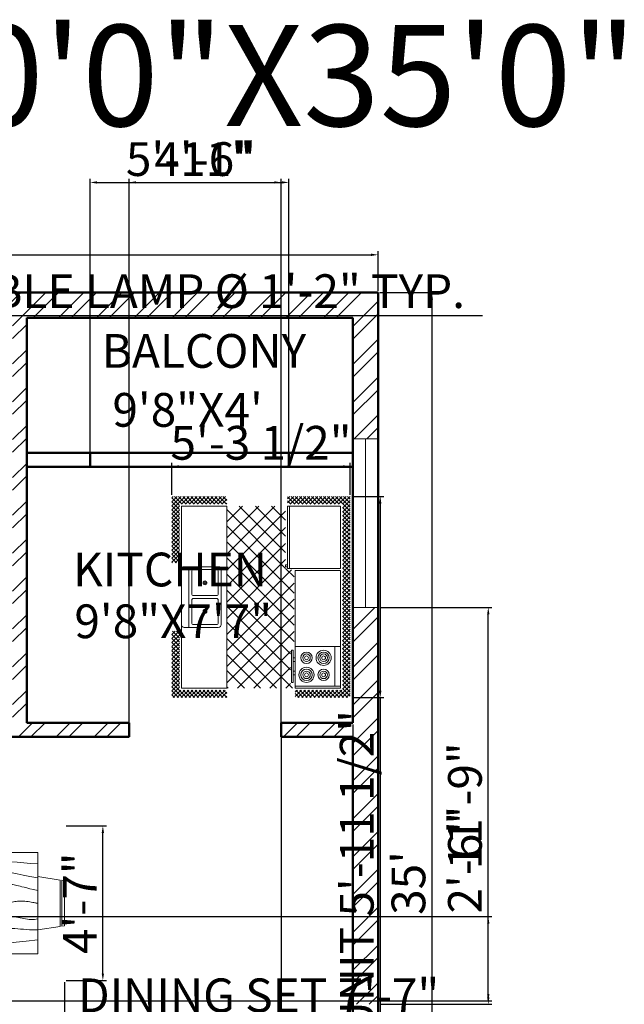
# Model space of a CAD drawing. Units: inches. Extents: x 1954 to 2815, y 1733 to 2371.
# Tile 4 of 4: x 2592 to 2807, y 2012 to 2362. Entities that reach past the tile are written whole.
import ezdxf

# ---------------------------------------------------------------- set-up
doc = ezdxf.new("R2010")
doc.units = ezdxf.units.IN
for name, color, linetype, lineweight in [('A-ANNO-DIMS', 2, 'Continuous', 18), ('A-ANNO-TEXT', 7, 'Continuous', 25), ('A-AREA-IDEN', 7, 'Continuous', 25), ('A-FLOR-FIXT', 9, 'Continuous', 20), ('A-FURN', 8, 'Continuous', 18), ('A-GLAZ', 4, 'Continuous', 18), ('A-WALL', 7, 'Continuous', 50), ('A-WALL-PATT', 252, 'Continuous', 13)]:
    doc.layers.add(name, color=color, linetype=linetype, lineweight=lineweight)
doc.styles.get("Standard").update_dxf_attribs({"font": 'arial.ttf'})
doc.dimstyles.new('ISO-25', dxfattribs={"dimtxt": 12, "dimasz": 2.5, "dimexe": 1.25, "dimexo": 0.625, "dimtad": 1, "dimdec": 1, "dimlunit": 4, "dimtxsty": 'Standard', "dimcen": 2.5, "dimadec": 0, "dimazin": 0, "dimtfac": 1, "dimtdec": 1, "dimtmove": 0, "dimatfit": 3, "dimfxl": 1, "dimarcsym": 0})

# ---------------------------------------------------------------- blocks, each defined once
blk = doc.blocks.new('Kitchen Layout - 7 x 8 ft')
for p, q in [((-5, 81.32), (2.68, 89)), ((-5, 83.44), (0.56, 89)), ((-5, 85.56), (-1.56, 89)), ((-5, 87.68), (-3.68, 89)), ((-1, 84.97), (-5, 88.97)), ((1.09, 85), (-2.91, 89)), ((3.21, 85), (-0.79, 89)), ((0.81, 85), (4.81, 89)), ((5.34, 85), (1.34, 89)), ((2.93, 85), (6.93, 89)), ((7.46, 85), (3.46, 89)), ((5.05, 85), (9.05, 89)), ((9.58, 85), (5.58, 89)), ((7.17, 85), (11.17, 89)), ((11.7, 85), (7.7, 89)), ((9.29, 85), (13.29, 89)), ((13.82, 85), (9.82, 89)), ((11.41, 85), (15.41, 89)), ((15.94, 85), (11.94, 89)), ((13.53, 85), (17.53, 89)), ((18.06, 85), (14.06, 89)), ((15.65, 85), (19.65, 89)), ((20.18, 85), (16.18, 89)), ((17.78, 85), (21.78, 89)), ((22.31, 85), (18.31, 89)), ((19.9, 85), (23.9, 89)), ((24.43, 85), (20.43, 89)), ((22.02, 85), (26.02, 89)), ((26.55, 85), (22.55, 89)), ((24.14, 85), (28.14, 89)), ((28.67, 85), (24.67, 89)), ((26.26, 85), (30.26, 89)), ((30.79, 85), (26.79, 89)), ((28.38, 85), (32.38, 89)), ((32.91, 85), (28.91, 89)), ((30.5, 85), (34.5, 89)), ((35.03, 85), (31.03, 89)), ((32.63, 85), (36.63, 89)), ((37.16, 85), (33.16, 89)), ((34.75, 85), (38.75, 89)), ((39.28, 85), (35.28, 89)), ((36.87, 85), (40.87, 89)), ((41.4, 85), (37.4, 89)), ((38.99, 85), (42.99, 89)), ((43.52, 85), (39.52, 89)), ((41.11, 85), (45.11, 89)), ((45.64, 85), (41.64, 89)), ((43.23, 85), (47.23, 89)), ((47.76, 85), (43.76, 89)), ((45.35, 85), (49.35, 89)), ((49.88, 85), (45.88, 89)), ((47.47, 85), (51.47, 89)), ((52, 85), (48, 89)), ((49.6, 85), (53.6, 89)), ((54.13, 85), (50.13, 89)), ((51.72, 85), (55.72, 89)), ((56.25, 85), (52.25, 89)), ((53.84, 85), (57.84, 89)), ((58.37, 85), (54.37, 89)), ((55.96, 85), (59.96, 89)), ((60.49, 85), (56.49, 89)), ((58.08, 85), (62.08, 89)), ((62.61, 85), (58.61, 89)), ((60.2, 85), (64.2, 89)), ((64.73, 85), (60.73, 89)), ((62.32, 85), (66.32, 89)), ((66.85, 85), (62.85, 89)), ((64.45, 85), (68.45, 89)), ((68.97, 85), (64.97, 89)), ((66.57, 85), (70.57, 89)), ((71.1, 85), (67.1, 89)), ((68.69, 85), (72.69, 89)), ((73.22, 85), (69.22, 89)), ((70.81, 85), (74.81, 89)), ((75.34, 85), (71.34, 89)), ((72.93, 85), (76.93, 89)), ((77.46, 85), (73.46, 89)), ((75.05, 85), (79.05, 89)), ((79.58, 85), (75.58, 89)), ((77.17, 85), (81.17, 89)), ((81.7, 85), (77.7, 89)), ((79.29, 85), (83.29, 89)), ((83.82, 85), (79.82, 89)), ((81.42, 85), (85.42, 89)), ((85.95, 85), (81.95, 89)), ((83.54, 85), (87.54, 89)), ((88.07, 85), (84.07, 89)), ((85.66, 85), (89.66, 89)), ((90.19, 85), (86.19, 89)), ((87.78, 85), (91.78, 89)), ((92.31, 85), (88.31, 89)), ((89.9, 85), (93.9, 89)), ((94.43, 85), (90.43, 89)), ((92.02, 85), (96.02, 89)), ((96.55, 85), (92.55, 89)), ((94.14, 85), (98.14, 89)), ((101, 82.67), (94.67, 89)), ((96.27, 85), (100.27, 89)), ((101, 84.79), (96.79, 89)), ((101, 86.92), (98.92, 89)), ((-1, 82.85), (-5, 86.85)), ((-1, 80.73), (-5, 84.73)), ((-5, 79.19), (-1, 83.19)), ((34, 84), (96, 84)), ((34, 60), (34, 84)), ((96, 84), (96, 60)), ((97, 83.61), (101, 87.61)), ((97, 81.49), (101, 85.49)), ((101, 80.55), (97, 84.55)), ((97, 79.37), (101, 83.37)), ((-1, 78.61), (-5, 82.61)), ((-5, 77.07), (-1, 81.07)), ((-1, 76.49), (-5, 80.49)), ((-5, 74.95), (-1, 78.95)), ((-1, 74.36), (-5, 78.36)), ((74, 81), (95, 81)), ((101, 78.43), (97, 82.43)), ((97, 77.25), (101, 81.25)), ((101, 76.31), (97, 80.31)), ((97, 75.13), (101, 79.13)), ((101, 74.19), (97, 78.19)), ((-5, 72.83), (-1, 76.83)), ((-1, 72.24), (-5, 76.24)), ((-5, 70.71), (-1, 74.71)), ((-1, 70.12), (-5, 74.12)), ((97, 73.01), (101, 77.01)), ((101, 72.07), (97, 76.07)), ((97, 70.89), (101, 74.89)), ((101, 69.95), (97, 73.95)), ((97, 68.76), (101, 72.76)), ((-5, 68.59), (-1, 72.59)), ((-1, 68), (-5, 72)), ((-5, 66.47), (-1, 70.47)), ((-1, 65.88), (-5, 69.88)), ((-5, 64.35), (-1, 68.35)), ((-1, 63.76), (-5, 67.76)), ((101, 67.82), (97, 71.82)), ((97, 66.64), (101, 70.64)), ((101, 65.7), (97, 69.7)), ((97, 64.52), (101, 68.52)), ((101, 63.58), (97, 67.58)), ((-5, 62.22), (-1, 66.22)), ((-1, 61.64), (-5, 65.64)), ((-5, 60.1), (-1, 64.1)), ((-1, 59.52), (-5, 63.52)), ((97, 62.4), (101, 66.4)), ((101, 61.46), (97, 65.46)), ((97, 60.28), (101, 64.28)), ((100.34, 60), (97, 63.34)), ((-5, 57.98), (-1, 61.98)), ((-1, 57.39), (-5, 61.39)), ((-1.73, 56), (-5, 59.27)), ((-3.85, 56), (-5, 57.15)), ((-4.86, 56), (-1, 59.86)), ((-2.74, 56), (-1, 57.74)), ((10.4, 24), (45.9, 59.5)), ((18.88, 24), (54.38, 59.5)), ((27.37, 24), (62.87, 59.5)), ((33.03, 55.11), (37.41, 59.5)), ((67.71, 24), (33.68, 58.04)), ((96, 60), (34, 60)), ((35.85, 24), (71.35, 59.5)), ((76.2, 24), (40.7, 59.5)), ((44.34, 24), (77.84, 57.5)), ((84.68, 24), (49.18, 59.5)), ((52.82, 24), (86.32, 57.5)), ((93.17, 24), (57.67, 59.5)), ((61.31, 24), (96, 58.69)), ((96, 29.65), (66.15, 59.5)), ((96, 38.14), (76.64, 57.5)), ((80, 60), (80, 59)), ((82, 59), (82, 60)), ((96, 46.63), (85.13, 57.5)), ((87, 59), (87, 60)), ((89, 60), (89, 59)), ((96, 55.11), (93.57, 57.54)), ((98.22, 60), (97, 61.22)), ((98.84, 60), (101, 62.16)), ((100.96, 60), (101, 60.04)), ((0, 57), (33, 57)), ((0, 30.57), (24.43, 55)), ((0, 39.06), (15.94, 55)), ((0, 47.54), (7.46, 55)), ((1.91, 24), (32.91, 55)), ((33.77, 24), (2.77, 55)), ((42.26, 24), (11.26, 55)), ((50.74, 24), (19.74, 55)), ((59.23, 24), (28.23, 55)), ((31, 55), (31, 56)), ((32, 55), (31, 55)), ((32, 56), (32, 55)), ((25.29, 24), (0, 49.29)), ((69.79, 24), (96, 50.21)), ((78.28, 24), (96, 41.72)), ((16.8, 24), (0, 40.8)), ((8.32, 24), (0, 32.32)), ((86.76, 24), (96, 33.24)), ((-5, 21.92), (-2.92, 24)), ((-5, 19.8), (-1, 23.8)), ((-1, 19.21), (-5, 23.21)), ((-5, 17.68), (-1, 21.68)), ((-1, 17.09), (-5, 21.09)), ((-1, 21.33), (-3.67, 24)), ((-1, 23.45), (-1.55, 24)), ((0, 24), (96, 24)), ((0, 0), (0, 24)), ((95.25, 24), (96, 24.75)), ((96, 24), (96, 0)), ((97, 22.1), (98.9, 24)), ((97, 19.97), (101, 23.97)), ((101, 19.03), (97, 23.03)), ((97, 17.85), (101, 21.85)), ((101, 16.91), (97, 20.91)), ((101, 21.16), (98.16, 24)), ((101, 23.28), (100.28, 24)), ((-5, 15.55), (-1, 19.55)), ((-1, 14.97), (-5, 18.97)), ((-5, 13.43), (-1, 17.43)), ((-1, 12.85), (-5, 16.85)), ((47.25, 6.5), (47.25, 18.5)), ((48.75, 18.5), (48.75, 6.5)), ((97, 15.73), (101, 19.73)), ((101, 14.79), (97, 18.79)), ((97, 13.61), (101, 17.61)), ((101, 12.67), (97, 16.67)), ((-5, 11.31), (-1, 15.31)), ((-1, 10.73), (-5, 14.73)), ((-5, 9.19), (-1, 13.19)), ((-1, 8.6), (-5, 12.6)), ((-5, 7.07), (-1, 11.07)), ((-1, 6.48), (-5, 10.48)), ((97, 11.49), (101, 15.49)), ((101, 10.55), (97, 14.55)), ((97, 9.37), (101, 13.37)), ((101, 8.43), (97, 12.43)), ((97, 7.25), (101, 11.25)), ((-5, 4.95), (-1, 8.95)), ((-1, 4.36), (-5, 8.36)), ((-5, 2.83), (-1, 6.83)), ((-1, 2.24), (-5, 6.24)), ((101, 6.31), (97, 10.31)), ((97, 5.12), (101, 9.12)), ((101, 4.18), (97, 8.18)), ((97, 3), (101, 7)), ((101, 2.06), (97, 6.06)), ((-5, 0.71), (-1, 4.71)), ((-1, 0.12), (-5, 4.12)), ((-5, -1.42), (-1, 2.58)), ((2, -5), (-5, 2)), ((-5, -3.54), (-1, 0.46)), ((96, 0), (0, 0)), ((64, 4), (32, 4)), ((93.24, -5), (101, 2.76)), ((95.36, -5), (101, 0.64)), ((97, 0.88), (101, 4.88)), ((101, -0.06), (97, 3.94)), ((101, -2.18), (97, 1.82)), ((-0.12, -5), (-5, -0.12)), ((-2.25, -5), (-5, -2.25)), ((-4.37, -5), (-5, -4.37)), ((-4.34, -5), (-0.34, -1)), ((-2.22, -5), (1.78, -1)), ((-0.1, -5), (3.9, -1)), ((4.12, -5), (0.12, -1)), ((2.02, -5), (6.02, -1)), ((6.24, -5), (2.24, -1)), ((4.14, -5), (8.14, -1)), ((8.36, -5), (4.36, -1)), ((6.27, -5), (10.27, -1)), ((10.48, -5), (6.48, -1)), ((8.39, -5), (12.39, -1)), ((12.6, -5), (8.6, -1)), ((10.51, -5), (14.51, -1)), ((14.73, -5), (10.73, -1)), ((12.63, -5), (16.63, -1)), ((16.85, -5), (12.85, -1)), ((14.75, -5), (18.75, -1)), ((18.97, -5), (14.97, -1)), ((16.87, -5), (20.87, -1)), ((21.09, -5), (17.09, -1)), ((18.99, -5), (22.99, -1)), ((23.21, -5), (19.21, -1)), ((21.11, -5), (25.11, -1)), ((25.33, -5), (21.33, -1)), ((23.24, -5), (27.24, -1)), ((27.45, -5), (23.45, -1)), ((25.36, -5), (29.36, -1)), ((29.57, -5), (25.57, -1)), ((27.48, -5), (30, -2.48)), ((30, -3.3), (27.7, -1)), ((29.6, -5), (30, -4.6)), ((30, -1.18), (29.82, -1)), ((66, -2.54), (67.54, -1)), ((66, -4.66), (69.66, -1)), ((69.88, -5), (66, -1.12)), ((67.76, -5), (66, -3.24)), ((67.78, -5), (71.78, -1)), ((72, -5), (68, -1)), ((69.9, -5), (73.9, -1)), ((74.12, -5), (70.12, -1)), ((72.03, -5), (76.03, -1)), ((76.24, -5), (72.24, -1)), ((74.15, -5), (78.15, -1)), ((78.36, -5), (74.36, -1)), ((76.27, -5), (80.27, -1)), ((80.49, -5), (76.49, -1)), ((78.39, -5), (82.39, -1)), ((82.61, -5), (78.61, -1)), ((80.51, -5), (84.51, -1)), ((84.73, -5), (80.73, -1)), ((82.63, -5), (86.63, -1)), ((86.85, -5), (82.85, -1)), ((84.75, -5), (88.75, -1)), ((88.97, -5), (84.97, -1)), ((86.88, -5), (90.88, -1)), ((91.09, -5), (87.09, -1)), ((89, -5), (93, -1)), ((93.21, -5), (89.21, -1)), ((91.12, -5), (95.12, -1)), ((95.34, -5), (91.34, -1)), ((97.46, -5), (93.46, -1)), ((99.58, -5), (95.58, -1)), ((101, -4.3), (97, -0.3)), ((97.48, -5), (101, -1.48)), ((99.6, -5), (101, -3.6))]:
    blk.add_line(p, q)
for points in [[(0, 56), (0, 84), (33, 84), (33, 56)], [(74, 60), (74, 84), (95, 84), (95, 60)], [(76, 58), (76, 59), (93, 59), (93, 58)]]:
    blk.add_lwpolyline(points, close=True)
for points in [[(33.5, 21), (62.5, 21)], [(32, 1.5), (32, 19.5)], [(33.5, 6.5), (33.5, 18.5)], [(34.5, 19.5), (46.25, 19.5)], [(49.75, 19.5), (61.5, 19.5)], [(62.5, 18.5), (62.5, 6.5)], [(64, 19.5), (64, 1.5)], [(46.25, 5.5), (34.5, 5.5)], [(61.5, 5.5), (49.75, 5.5)], [(62.5, 0), (33.5, 0)]]:
    blk.add_lwpolyline(points)
for centre, radius in [((80, 75), 4), ((80, 75), 3), ((89, 75), 3), ((80, 75), 2), ((80, 75), 1), ((89, 75), 2), ((89, 75), 1), ((80, 66), 3), ((80, 66), 2), ((89, 66), 4), ((89, 66), 3), ((89, 66), 2), ((80, 66), 1), ((89, 66), 1), ((40.5, 12.5), 1), ((40.5, 12.5), 0.5), ((55.5, 12.5), 1), ((55.5, 12.5), 0.5)]:
    blk.add_circle(centre, radius)
for centre, radius, start, end in [((33.5, 19.5), 1.5, 90, 180), ((62.5, 19.5), 1.5, 0, 90), ((34.5, 18.5), 1, 90, 180), ((46.25, 18.5), 1, 0, 90), ((49.75, 18.5), 1, 90, 180), ((61.5, 18.5), 1, 0, 90), ((34.5, 6.5), 1, 180, 270), ((46.25, 6.5), 1, 270, 0), ((49.75, 6.5), 1, 180, 270), ((61.5, 6.5), 1, 270, 0), ((33.5, 1.5), 1.5, 180, 270), ((62.5, 1.5), 1.5, 270, 0)]:
    blk.add_arc(centre, radius, start, end)
blk = doc.blocks.new('Dining Set - 36 x 72 in.')
for p, q in [((-22.2343, 26.00059), (-23.4847, 17.99762)), ((-22.2304, 26), (-5.7608, 26)), ((-22, 27.5), (-22.1562, 26.50042)), ((-5.8416, 26.5), (-22.1534, 26.5)), ((-22, 27.5), (-6, 27.5)), ((-5.8437, 26.49966), (-6, 27.5)), ((-4.5152, 17.99762), (-5.7655, 25.99926)), ((5.7657, 26.00059), (4.5153, 17.99762)), ((5.7696, 26), (22.2392, 26)), ((6, 27.5), (5.8438, 26.50042)), ((22.1584, 26.5), (5.8466, 26.5)), ((6, 27.5), (22, 27.5)), ((22.1563, 26.49966), (22, 27.5)), ((23.4848, 17.99762), (22.2345, 25.99926)), ((36, 18), (-36, 18)), ((-36, 18), (-36, -18)), ((36, -18), (36, 18)), ((-45.5, 8), (-44.5004, 8.15617)), ((-45.5, 8), (-45.5, -8)), ((-44.5, -8.15843), (-44.5, 8.15338)), ((-44.0006, 8.23428), (-35.9976, 9.48474)), ((-44, 8.23041), (-44, -8.23915)), ((44.0006, 8.23428), (35.9976, 9.48474)), ((44, 8.23041), (44, -8.23915)), ((44.5, -8.15843), (44.5, 8.15338)), ((45.5, 8), (44.5005, 8.15617)), ((45.5, 8), (45.5, -8)), ((-44.4997, -8.15631), (-45.5, -8)), ((-35.9976, -9.48476), (-43.9993, -8.2345)), ((35.9976, -9.48476), (43.9993, -8.2345)), ((44.4997, -8.15631), (45.5, -8)), ((-36, -18), (36, -18)), ((-22.2343, -26.0006), (-23.4847, -17.99762)), ((-4.5152, -17.99762), (-5.7655, -25.99928)), ((5.7657, -26.0006), (4.5153, -17.99762)), ((23.4848, -17.99762), (22.2345, -25.99928)), ((-22.2304, -26), (-5.7608, -26)), ((-22, -27.5), (-22.1562, -26.50044)), ((-5.8416, -26.5), (-22.1534, -26.5)), ((-22, -27.5), (-6, -27.5)), ((-5.8437, -26.49967), (-6, -27.5)), ((5.7696, -26), (22.2392, -26)), ((6, -27.5), (5.8438, -26.50044)), ((22.1584, -26.5), (5.8466, -26.5)), ((6, -27.5), (22, -27.5)), ((22.1563, -26.49967), (22, -27.5))]:
    blk.add_line(p, q)
for points in [[(-36, 15), (-31.1772, 14.97754), (-26.8079, 14.91406), (-22.8538, 14.81543), (-19.276, 14.6875), (-16.0362, 14.53613), (-13.0957, 14.36718), (-10.4159, 14.18652), (-7.9583, 14), (-5.6904, 13.81315), (-3.6035, 13.63021), (-1.6954, 13.45508), (0.0365, 13.29166), (1.5945, 13.14388), (2.9811, 13.01562), (4.1988, 12.9108), (5.25, 12.83333), (6.1393, 12.78613), (6.8802, 12.76823), (7.4883, 12.77767), (7.9792, 12.8125), (8.3685, 12.87077), (8.6719, 12.95052), (8.9049, 13.0498), (9.0833, 13.16666), (9.2205, 13.29899), (9.3216, 13.44401), (9.3895, 13.59879), (9.4271, 13.76041), (9.4373, 13.92594), (9.4232, 14.09245), (9.3875, 14.257), (9.3333, 14.41666), (9.2638, 14.56917), (9.1836, 14.71484), (9.0975, 14.85465), (9.0104, 14.98958), (8.9272, 15.1206), (8.8529, 15.2487), (8.7922, 15.37483), (8.75, 15.5), (8.7305, 15.62467), (8.7344, 15.74739), (8.7617, 15.86621), (8.8125, 15.97916), (8.8867, 16.08431), (8.9844, 16.17968), (9.1055, 16.26334), (9.25, 16.33333), (9.4189, 16.38802), (9.6172, 16.42708), (9.8506, 16.45052), (10.125, 16.45833), (10.4463, 16.45052), (10.8203, 16.42708), (11.2529, 16.38802), (11.75, 16.33333), (12.3184, 16.26318), (12.9694, 16.17838), (13.7151, 16.07991), (14.5677, 15.96875), (15.5395, 15.84586), (16.6426, 15.71224), (17.8893, 15.56884), (19.2917, 15.41666), (20.859, 15.25667), (22.5879, 15.08984), (24.4721, 14.91715), (26.5052, 14.73958), (28.6809, 14.5581), (30.9929, 14.3737), (33.4347, 14.18733), (36, 14)], [(-36, 10), (-28.9766, 10.14274), (-23.1725, 10.20442), (-18.4241, 10.19775), (-14.5677, 10.13541), (-11.4399, 10.03011), (-8.877, 9.89453), (-6.7154, 9.74137), (-4.7917, 9.58333), (-2.9698, 9.43082), (-1.2246, 9.28515), (0.4415, 9.14534), (2.026, 9.01041), (3.5266, 8.87939), (4.9408, 8.7513), (6.266, 8.62516), (7.5, 8.5), (8.6411, 8.37549), (9.6914, 8.2539), (10.6538, 8.13818), (11.5312, 8.03125), (12.3267, 7.93603), (13.043, 7.85547), (13.6831, 7.79248), (14.25, 7.75), (14.7471, 7.7303), (15.1797, 7.73307), (15.5537, 7.75732), (15.875, 7.80208), (16.1494, 7.86637), (16.3828, 7.94922), (16.5811, 8.04964), (16.75, 8.16666), (16.8944, 8.29915), (17.0143, 8.44531), (17.1089, 8.60319), (17.1771, 8.77083), (17.218, 8.94629), (17.2305, 9.1276), (17.2137, 9.31282), (17.1667, 9.5), (17.0895, 9.6875), (16.987, 9.875), (16.8649, 10.0625), (16.7292, 10.25), (16.5856, 10.4375), (16.4401, 10.625), (16.2985, 10.8125), (16.1667, 11), (16.05, 11.18733), (15.9518, 11.3737), (15.8752, 11.5581), (15.8229, 11.73958), (15.798, 11.91715), (15.8034, 12.08984), (15.842, 12.25667), (15.9167, 12.41666), (16.0295, 12.56836), (16.1784, 12.70833), (16.3605, 12.83268), (16.5729, 12.9375), (16.8127, 13.01888), (17.0768, 13.07291), (17.3625, 13.0957), (17.6667, 13.08333), (17.9894, 13.03312), (18.3418, 12.94726), (18.7382, 12.82918), (19.1927, 12.68229), (19.7195, 12.51001), (20.3327, 12.31575), (21.0465, 12.10294), (21.875, 11.875), (22.8357, 11.63354), (23.959, 11.37304), (25.2786, 11.08618), (26.8282, 10.76562), (28.6414, 10.40405), (30.752, 9.99414), (33.1936, 9.52856), (36, 9)], [(-36, 5.5), (-30.7157, 5.3348), (-26.069, 5.20963), (-21.9946, 5.11767), (-18.4271, 5.05208), (-15.3009, 5.00602), (-12.5508, 4.97265), (-10.1112, 4.94515), (-7.9167, 4.91666), (-5.909, 4.88167), (-4.0586, 4.83984), (-2.3429, 4.79215), (-0.7396, 4.73958), (0.7739, 4.6831), (2.22, 4.6237), (3.6213, 4.56233), (5, 4.5), (6.373, 4.43782), (7.7344, 4.3776), (9.0723, 4.32129), (10.375, 4.27083), (11.6309, 4.22819), (12.8281, 4.19531), (13.9551, 4.17415), (15, 4.16666), (15.954, 4.17448), (16.819, 4.19791), (17.6001, 4.23698), (18.3021, 4.29166), (18.9299, 4.36198), (19.4883, 4.44791), (19.9823, 4.54948), (20.4167, 4.66666), (20.7969, 4.79899), (21.1302, 4.94401), (21.4245, 5.09879), (21.6875, 5.26041), (21.9271, 5.42594), (22.1511, 5.59245), (22.3672, 5.757), (22.5834, 5.91666), (22.8065, 6.06868), (23.0404, 6.21093), (23.2879, 6.34147), (23.5521, 6.45833), (23.8358, 6.55957), (24.142, 6.64323), (24.4735, 6.70735), (24.8334, 6.75), (25.2235, 6.76969), (25.642, 6.76692), (26.0858, 6.74267), (26.5521, 6.69791), (27.0379, 6.63362), (27.5404, 6.55078), (28.0565, 6.45036), (28.5834, 6.33333), (29.1242, 6.19987), (29.7071, 6.04687), (30.3661, 5.87044), (31.1354, 5.66666), (32.0493, 5.43164), (33.142, 5.16146), (34.4475, 4.85221), (36, 4.5)], [(-36, -1), (-30.7915, -0.6591), (-26.0195, -0.38216), (-21.6519, -0.16284), (-17.6563, 0.00521), (-14.0005, 0.12833), (-10.6523, 0.21289), (-7.5796, 0.26522), (-4.75, 0.29166), (-2.134, 0.29793), (0.2878, 0.28711), (2.5317, 0.26163), (4.6146, 0.22396), (6.5529, 0.17651), (8.3633, 0.12174), (10.0623, 0.06209), (11.6667, 0), (13.1899, -0.06201), (14.6341, -0.1211), (15.9982, -0.17432), (17.2813, -0.21875), (18.4823, -0.25147), (19.6003, -0.26953), (20.6343, -0.27002), (21.5834, -0.25), (22.4481, -0.20768), (23.2357, -0.14584), (23.9549, -0.06836), (24.6146, 0.02083), (25.2235, 0.11784), (25.7904, 0.21875), (26.3241, 0.31966), (26.8334, 0.41666), (27.3265, 0.50618), (27.8099, 0.58593), (28.2894, 0.65397), (28.7709, 0.70833), (29.2601, 0.74707), (29.763, 0.76823), (30.2855, 0.76985), (30.8334, 0.75), (31.4088, 0.70784), (31.9994, 0.64713), (32.589, 0.57275), (33.1615, 0.48958), (33.7008, 0.4025), (34.1908, 0.3164), (34.6153, 0.23616), (34.9584, 0.16666), (35.2099, 0.11165), (35.3848, 0.07031), (35.504, 0.04069), (35.5886, 0.02083), (35.6594, 0.00879), (35.7377, 0.0026), (35.8442, 0.00032), (36, 0)], [(-36, -6.5), (-27.1843, -6.31267), (-20.084, -6.1263), (-14.469, -5.9419), (-10.1094, -5.76042), (-6.7752, -5.58285), (-4.2363, -5.41016), (-2.2629, -5.24333), (-0.625, -5.08334), (0.8708, -4.93099), (2.2715, -4.78646), (3.5872, -4.64974), (4.8281, -4.52084), (6.0046, -4.39974), (7.127, -4.28646), (8.2053, -4.18099), (9.25, -4.08334), (10.2705, -3.99382), (11.2734, -3.91407), (12.2647, -3.84603), (13.25, -3.79167), (14.2354, -3.75293), (15.2266, -3.73177), (16.2295, -3.73015), (17.25, -3.75), (18.2912, -3.79248), (19.3451, -3.85547), (20.4009, -3.93604), (21.4479, -4.03125), (22.4754, -4.13819), (23.4727, -4.25391), (24.4289, -4.37549), (25.3334, -4.5), (26.1785, -4.62492), (26.9694, -4.74935), (27.7145, -4.87281), (28.4219, -4.99479), (29.1, -5.11483), (29.7572, -5.23242), (30.4016, -5.34709), (31.0417, -5.45834), (31.6837, -5.56437), (32.3262, -5.65821), (32.9658, -5.73153), (33.599, -5.77604), (34.2224, -5.78345), (34.8327, -5.74545), (35.4264, -5.65373), (36, -5.5)], [(-36, -10), (-26.4022, -9.81299), (-18.4675, -9.62891), (-11.9839, -9.45069), (-6.7396, -9.28125), (-2.5226, -9.12354), (0.8789, -8.98047), (3.6769, -8.85498), (6.0833, -8.75), (8.2767, -8.66765), (10.3021, -8.60677), (12.1712, -8.56543), (13.8958, -8.54167), (15.4876, -8.53353), (16.9583, -8.53907), (18.3197, -8.55632), (19.5834, -8.58334), (20.7616, -8.61841), (21.8685, -8.66081), (22.9188, -8.71004), (23.9271, -8.76563), (24.9081, -8.82707), (25.8763, -8.89388), (26.8465, -8.96558), (27.8334, -9.04167), (28.8474, -9.12118), (29.8828, -9.20117), (30.93, -9.27824), (31.9792, -9.34896), (33.0205, -9.40991), (34.0443, -9.45768), (35.0407, -9.48885), (36, -9.5)], [(-36, -14.5), (-30.0881, -14.33513), (-25.0332, -14.21224), (-20.7312, -14.12647), (-17.0781, -14.07292), (-13.97, -14.04671), (-11.3027, -14.04297), (-8.9724, -14.05681), (-6.875, -14.08334), (-4.9224, -14.11833), (-3.0905, -14.16016), (-1.3709, -14.20785), (0.2448, -14.26042), (1.7647, -14.3169), (3.1973, -14.3763), (4.5507, -14.43767), (5.8333, -14.5), (7.0554, -14.5621), (8.235, -14.62175), (9.3922, -14.67652), (10.5469, -14.72396), (11.7192, -14.76164), (12.929, -14.78711), (14.1965, -14.79794), (15.5417, -14.79167), (16.9933, -14.76424), (18.6152, -14.70508), (20.4804, -14.60197), (22.6615, -14.44271), (25.2312, -14.21509), (28.2624, -13.9069), (31.8277, -13.50594), (36, -13)]]:
    blk.add_lwpolyline(points)
blk = doc.blocks.new('*D10')
at = {"layer": 'A-ANNO-DIMS', "color": 0, "lineweight": -2, "transparency": 16777216}
for p, q in [((2239.88, 2265.61), (2239.88, 2279.68)), ((2242.38, 2278.43), (2717.38, 2278.43)), ((2719.88, 2265.61), (2719.88, 2279.68))]:
    blk.add_line(p, q, dxfattribs=at)
at = {"layer": 'A-ANNO-DIMS', "color": 0, "transparency": 16777216}
for points in [[(2242.38, 2278.85), (2242.38, 2278.01), (2239.88, 2278.43)], [(2717.38, 2278.85), (2717.38, 2278.01), (2719.88, 2278.43)]]:
    blk.add_solid(points, dxfattribs=at)
at = {"layer": 'Defpoints', "color": 0, "transparency": 16777216}
for p in [(2719.88, 2278.43), (2239.88, 2264.98), (2719.88, 2264.98)]:
    blk.add_point(p, dxfattribs=at)
at = {"layer": 'A-ANNO-DIMS', "color": 0, "transparency": 16777216, "insert": (2479.88, 2285.18), "char_height": 12, "attachment_point": 5}
blk.add_mtext("40'", dxfattribs=at)
blk = doc.blocks.new('*D11')
at = {"layer": 'A-ANNO-DIMS', "color": 0, "lineweight": -2, "transparency": 16777216}
for p, q in [((2720.51, 2264.98), (2740.24, 2264.98)), ((2738.99, 2262.48), (2738.99, 1847.48)), ((2720.51, 1844.98), (2740.24, 1844.98))]:
    blk.add_line(p, q, dxfattribs=at)
at = {"layer": 'A-ANNO-DIMS', "color": 0, "transparency": 16777216}
for points in [[(2738.57, 2262.48), (2739.41, 2262.48), (2738.99, 2264.98)], [(2738.57, 1847.48), (2739.41, 1847.48), (2738.99, 1844.98)]]:
    blk.add_solid(points, dxfattribs=at)
at = {"layer": 'Defpoints', "color": 0, "transparency": 16777216}
for p in [(2719.88, 2264.98), (2719.88, 1844.98), (2738.99, 1844.98)]:
    blk.add_point(p, dxfattribs=at)
at = {"layer": 'A-ANNO-DIMS', "color": 0, "transparency": 16777216, "insert": (2732.23, 2054.98), "char_height": 12, "attachment_point": 5, "rotation": 90}
blk.add_mtext("35'", dxfattribs=at)
blk = doc.blocks.new('WIN-60IN')
blk.add_line((4.5, 60), (4.5, 0))
blk.add_lwpolyline([(9, 60), (9, 0), (0, 0), (0, 60)], close=True)
blk = doc.blocks.new('*D16')
at = {"layer": 'A-ANNO-DIMS', "color": 0, "lineweight": -2, "transparency": 16777216}
for p, q in [((2540.09, 2255.38), (2540.09, 2258.1)), ((2542.59, 2256.85), (2551.59, 2256.85)), ((2554.09, 2255.38), (2554.09, 2258.1)), ((2554.09, 2256.85), (2757.06, 2256.85))]:
    blk.add_line(p, q, dxfattribs=at)
at = {"layer": 'A-ANNO-DIMS', "color": 0, "transparency": 16777216}
for points in [[(2542.59, 2257.27), (2542.59, 2256.44), (2540.09, 2256.85)], [(2551.59, 2257.27), (2551.59, 2256.44), (2554.09, 2256.85)]]:
    blk.add_solid(points, dxfattribs=at)
at = {"layer": 'Defpoints', "color": 0, "transparency": 16777216}
for p in [(2554.09, 2256.85), (2540.09, 2254.75), (2554.09, 2254.75)]:
    blk.add_point(p, dxfattribs=at)
at = {"layer": 'A-ANNO-DIMS', "color": 0, "transparency": 16777216, "insert": (2656.83, 2263.94), "char_height": 12, "attachment_point": 5}
blk.add_mtext('TABLE LAMP Ø 1\'-2" TYP.', dxfattribs=at)
blk = doc.blocks.new('*D22')
at = {"layer": 'A-ANNO-DIMS', "color": 0, "lineweight": -2, "transparency": 16777216}
for p, q in [((2710.56, 2192.43), (2721.92, 2192.43)), ((2720.67, 2189.93), (2720.67, 2123.41)), ((2710.56, 2120.91), (2721.92, 2120.91)), ((2720.67, 2120.91), (2720.67, 1926.5))]:
    blk.add_line(p, q, dxfattribs=at)
at = {"layer": 'A-ANNO-DIMS', "color": 0, "transparency": 16777216}
for points in [[(2720.25, 2189.93), (2721.08, 2189.93), (2720.67, 2192.43)], [(2720.25, 2123.41), (2721.08, 2123.41), (2720.67, 2120.91)]]:
    blk.add_solid(points, dxfattribs=at)
at = {"layer": 'Defpoints', "color": 0, "transparency": 16777216}
for p in [(2709.94, 2192.43), (2709.94, 2120.91), (2720.67, 2120.91)]:
    blk.add_point(p, dxfattribs=at)
at = {"layer": 'A-ANNO-DIMS', "color": 0, "transparency": 16777216, "insert": (2713.84, 2022.46), "char_height": 12, "attachment_point": 5, "rotation": 90}
blk.add_mtext('KITCHEN UNIT 5\'-11 1/2"', dxfattribs=at)
blk = doc.blocks.new('*D23')
at = {"layer": 'A-ANNO-DIMS', "color": 0, "lineweight": -2, "transparency": 16777216}
for p, q in [((2646.51, 2193.06), (2646.51, 2204.41)), ((2709.94, 2193.06), (2709.94, 2204.41)), ((2649.01, 2203.16), (2707.44, 2203.16))]:
    blk.add_line(p, q, dxfattribs=at)
at = {"layer": 'A-ANNO-DIMS', "color": 0, "transparency": 16777216}
for points in [[(2649.01, 2203.58), (2649.01, 2202.75), (2646.51, 2203.16)], [(2707.44, 2203.58), (2707.44, 2202.75), (2709.94, 2203.16)]]:
    blk.add_solid(points, dxfattribs=at)
at = {"layer": 'Defpoints', "color": 0, "transparency": 16777216}
for p in [(2709.94, 2203.16), (2646.51, 2192.43), (2709.94, 2192.43)]:
    blk.add_point(p, dxfattribs=at)
at = {"layer": 'A-ANNO-DIMS', "color": 0, "transparency": 16777216, "insert": (2678.23, 2210), "char_height": 12, "attachment_point": 5}
blk.add_mtext('5\'-3 1/2"', dxfattribs=at)
blk = doc.blocks.new('*D24')
at = {"layer": 'A-ANNO-DIMS', "color": 0, "lineweight": -2, "transparency": 16777216}
for p, q in [((2517.32, 2019.64), (2517.32, 2005.36)), ((2608.32, 2019.64), (2608.32, 2005.36)), ((2519.82, 2006.61), (2605.82, 2006.61)), ((2608.32, 2006.61), (2743.97, 2006.61))]:
    blk.add_line(p, q, dxfattribs=at)
at = {"layer": 'A-ANNO-DIMS', "color": 0, "transparency": 16777216}
for points in [[(2519.82, 2007.03), (2519.82, 2006.2), (2517.32, 2006.61)], [(2605.82, 2007.03), (2605.82, 2006.2), (2608.32, 2006.61)]]:
    blk.add_solid(points, dxfattribs=at)
at = {"layer": 'Defpoints', "color": 0, "transparency": 16777216}
for p in [(2517.32, 2020.26), (2608.32, 2020.26), (2608.32, 2006.61)]:
    blk.add_point(p, dxfattribs=at)
at = {"layer": 'A-ANNO-DIMS', "color": 0, "transparency": 16777216, "insert": (2677.39, 2013.44), "char_height": 12, "attachment_point": 5}
blk.add_mtext('DINING SET 7\'-7"', dxfattribs=at)
blk = doc.blocks.new('*D25')
at = {"layer": 'A-ANNO-DIMS', "color": 0, "lineweight": -2, "transparency": 16777216}
for p, q in [((2608.95, 2075.26), (2623.22, 2075.26)), ((2621.97, 2022.76), (2621.97, 2072.76)), ((2608.95, 2020.26), (2623.22, 2020.26))]:
    blk.add_line(p, q, dxfattribs=at)
at = {"layer": 'A-ANNO-DIMS', "color": 0, "transparency": 16777216}
for points in [[(2621.56, 2072.76), (2622.39, 2072.76), (2621.97, 2075.26)], [(2621.56, 2022.76), (2622.39, 2022.76), (2621.97, 2020.26)]]:
    blk.add_solid(points, dxfattribs=at)
at = {"layer": 'Defpoints', "color": 0, "transparency": 16777216}
for p in [(2608.32, 2075.26), (2621.97, 2075.26), (2608.32, 2020.26)]:
    blk.add_point(p, dxfattribs=at)
at = {"layer": 'A-ANNO-DIMS', "color": 0, "transparency": 16777216, "insert": (2615.35, 2047.76), "char_height": 12, "attachment_point": 5, "rotation": 90}
blk.add_mtext('4\'-7"', dxfattribs=at)
blk = doc.blocks.new('*D45')
at = {"layer": 'A-ANNO-DIMS', "color": 0, "lineweight": -2, "transparency": 16777216}
for p, q in [((2720.51, 2153), (2760.33, 2153)), ((2759.08, 2014.3), (2759.08, 2150.5)), ((2720.51, 2011.8), (2760.33, 2011.8))]:
    blk.add_line(p, q, dxfattribs=at)
at = {"layer": 'A-ANNO-DIMS', "color": 0, "transparency": 16777216}
for points in [[(2758.67, 2150.5), (2759.5, 2150.5), (2759.08, 2153)], [(2758.67, 2014.3), (2759.5, 2014.3), (2759.08, 2011.8)]]:
    blk.add_solid(points, dxfattribs=at)
at = {"layer": 'Defpoints', "color": 0, "transparency": 16777216}
for p in [(2719.88, 2153), (2759.08, 2153), (2719.88, 2011.8)]:
    blk.add_point(p, dxfattribs=at)
at = {"layer": 'A-ANNO-DIMS', "color": 0, "transparency": 16777216, "insert": (2752.33, 2082.4), "char_height": 12, "attachment_point": 5, "rotation": 90}
blk.add_mtext('11\'-9"', dxfattribs=at)
blk = doc.blocks.new('*D50')
at = {"layer": 'A-ANNO-DIMS', "color": 0, "lineweight": -2, "transparency": 16777216}
for p, q in [((2631.3, 2107.61), (2631.3, 2305.43)), ((2685.45, 2107.61), (2685.45, 2305.43)), ((2633.8, 2304.18), (2682.95, 2304.18))]:
    blk.add_line(p, q, dxfattribs=at)
at = {"layer": 'A-ANNO-DIMS', "color": 0, "transparency": 16777216}
for points in [[(2633.8, 2304.6), (2633.8, 2303.77), (2631.3, 2304.18)], [(2682.95, 2304.6), (2682.95, 2303.77), (2685.45, 2304.18)]]:
    blk.add_solid(points, dxfattribs=at)
at = {"layer": 'Defpoints', "color": 0, "transparency": 16777216}
for p in [(2685.45, 2304.18), (2631.3, 2106.98), (2685.45, 2106.98)]:
    blk.add_point(p, dxfattribs=at)
at = {"layer": 'A-ANNO-DIMS', "color": 0, "transparency": 16777216, "insert": (2658.38, 2310.93), "char_height": 12, "attachment_point": 5}
blk.add_mtext('4\'-6"', dxfattribs=at)
blk = doc.blocks.new('*D51')
at = {"layer": 'A-ANNO-DIMS', "color": 0, "lineweight": -2, "transparency": 16777216}
for p, q in [((2685.45, 2111.36), (2685.45, 1768.53)), ((2710.88, 2111.36), (2710.88, 1768.53)), ((2687.95, 1769.78), (2708.38, 1769.78)), ((2710.88, 1769.78), (2774.7, 1769.78))]:
    blk.add_line(p, q, dxfattribs=at)
at = {"layer": 'A-ANNO-DIMS', "color": 0, "transparency": 16777216}
for points in [[(2687.95, 1770.2), (2687.95, 1769.37), (2685.45, 1769.78)], [(2708.38, 1770.2), (2708.38, 1769.37), (2710.88, 1769.78)]]:
    blk.add_solid(points, dxfattribs=at)
at = {"layer": 'Defpoints', "color": 0, "transparency": 16777216}
for p in [(2685.45, 2111.98), (2710.88, 2111.98), (2710.88, 1769.78)]:
    blk.add_point(p, dxfattribs=at)
at = {"layer": 'A-ANNO-DIMS', "color": 0, "transparency": 16777216, "insert": (2744.04, 1776.61), "char_height": 12, "attachment_point": 5}
blk.add_mtext('2\'-1 1/2"', dxfattribs=at)
blk = doc.blocks.new('*D52')
at = {"layer": 'A-ANNO-DIMS', "color": 0, "lineweight": -2, "transparency": 16777216}
for p, q in [((2759.08, 2043), (2759.08, 2078.85)), ((2344.56, 2043), (2760.33, 2043)), ((2759.08, 2015.5), (2759.08, 2040.5)), ((2344.56, 2013), (2760.33, 2013))]:
    blk.add_line(p, q, dxfattribs=at)
at = {"layer": 'A-ANNO-DIMS', "color": 0, "transparency": 16777216}
for points in [[(2758.67, 2040.5), (2759.5, 2040.5), (2759.08, 2043)], [(2758.67, 2015.5), (2759.5, 2015.5), (2759.08, 2013)]]:
    blk.add_solid(points, dxfattribs=at)
at = {"layer": 'Defpoints', "color": 0, "transparency": 16777216}
for p in [(2343.94, 2043), (2759.08, 2043), (2343.94, 2013)]:
    blk.add_point(p, dxfattribs=at)
at = {"layer": 'A-ANNO-DIMS', "color": 0, "transparency": 16777216, "insert": (2752.33, 2062.18), "char_height": 12, "attachment_point": 5, "rotation": 90}
blk.add_mtext('2\'-6"', dxfattribs=at)
blk = doc.blocks.new('*D56')
at = {"layer": 'A-ANNO-DIMS', "color": 0, "lineweight": -2, "transparency": 16777216}
for p, q in [((2617.4, 2203.61), (2617.4, 2305.43)), ((2688.16, 2203.61), (2688.16, 2305.43)), ((2619.9, 2304.18), (2685.66, 2304.18))]:
    blk.add_line(p, q, dxfattribs=at)
at = {"layer": 'A-ANNO-DIMS', "color": 0, "transparency": 16777216}
for points in [[(2619.9, 2304.6), (2619.9, 2303.77), (2617.4, 2304.18)], [(2685.66, 2304.6), (2685.66, 2303.77), (2688.16, 2304.18)]]:
    blk.add_solid(points, dxfattribs=at)
at = {"layer": 'Defpoints', "color": 0, "transparency": 16777216}
for p in [(2688.16, 2304.18), (2617.4, 2202.98), (2688.16, 2202.98)]:
    blk.add_point(p, dxfattribs=at)
at = {"layer": 'A-ANNO-DIMS', "color": 0, "transparency": 16777216, "insert": (2652.78, 2310.93), "char_height": 12, "attachment_point": 5}
blk.add_mtext('5\'-11"', dxfattribs=at)

msp = doc.modelspace()

# ---------------------------------------------------------------- hatches: boundary and pattern name
at = {"layer": 'A-WALL-PATT'}
h = msp.add_hatch(dxfattribs=at)
h.set_pattern_fill('ANSI32', color=256)
h.paths.add_polyline_path([(2480.43, 2264.98), (2354.46, 2264.98), (2354.46, 2255.98), (2416.88, 2255.98), (2416.88, 2111.98), (2405.35, 2111.98, -0.004167), (2405.36, 2111.48), (2405.36, 2106.98), (2487.77, 2106.98), (2487.77, 2111.48), (2487.77, 2111.98), (2421.88, 2111.98), (2421.88, 2255.98), (2480.43, 2255.98)])
h.paths.add_polyline_path([(2719.88, 2264.98), (2540.43, 2264.98), (2540.43, 2255.98), (2589.88, 2255.98), (2589.88, 2111.98), (2517.77, 2111.98, -0.004167), (2517.77, 2111.48), (2517.77, 2106.98), (2631.3, 2106.98), (2631.3, 2111.98), (2594.88, 2111.98), (2594.88, 2255.98), (2710.88, 2255.98), (2710.88, 2213), (2719.88, 2213)])
h = msp.add_hatch(dxfattribs=at)
h.set_pattern_fill('ANSI32', color=256)
h.paths.add_polyline_path([(2719.88, 2153), (2710.88, 2153), (2710.88, 2111.98), (2685.45, 2111.98), (2685.45, 2106.98), (2710.88, 2106.98), (2710.88, 2011.8), (2719.88, 2011.8)])

# ---------------------------------------------------------------- linework, layer by layer
at = {"layer": 'A-WALL'}
for p, q in [((2239.88, 2264.98), (2719.88, 2264.98)), ((2719.88, 2264.98), (2719.88, 1844.98)), ((2594.88, 2111.98), (2594.88, 2255.98)), ((2594.88, 2255.98), (2710.88, 2255.98)), ((2710.88, 2255.98), (2710.88, 2111.98)), ((2594.88, 2207.98), (2710.88, 2207.98)), ((2617.4, 2207.98), (2617.4, 2202.98)), ((2688.16, 2207.98), (2688.16, 2202.98)), ((2594.88, 2202.98), (2710.88, 2202.98)), ((2594.88, 2111.98), (2631.3, 2111.98)), ((2631.3, 2106.98), (2631.3, 2111.98)), ((2685.45, 2106.98), (2685.45, 2111.98)), ((2685.45, 2111.98), (2710.88, 2111.98)), ((2343.88, 2106.98), (2631.3, 2106.98)), ((2685.45, 2106.98), (2710.88, 2106.98)), ((2710.88, 2106.98), (2710.88, 1853.98))]:
    msp.add_line(p, q, dxfattribs=at)

# ---------------------------------------------------------------- block references
at = {"layer": 'A-FLOR-FIXT', "xscale": 0.6747450604021418, "yscale": 0.6747450604021418, "zscale": 0.6747450604021418, "rotation": 270}
msp.add_blockref('Kitchen Layout - 7 x 8 ft', (2649.89, 2189.06), dxfattribs=at)
at = {"layer": 'A-FURN'}
msp.add_blockref('Dining Set - 36 x 72 in.', (2562.82, 2047.76), dxfattribs=at)
at = {"layer": 'A-GLAZ'}
msp.add_blockref('WIN-60IN', (2710.88, 2153), dxfattribs=at)

# ---------------------------------------------------------------- texts
at = {"layer": 'A-ANNO-TEXT'}
msp.add_text('3BHK HOUSE PLAN 40\'0"X35\'0"', height=36, dxfattribs=at).set_placement((2097.45, 2324.21))
at = {"layer": 'A-AREA-IDEN'}
for s, p in [('BALCONY', (2621.56, 2238.24)), ('9\'8"X4\'', (2625.37, 2217.27)), ('KITCHEN', (2611.38, 2160.48)), ('9\'8"X7\'7"', (2611.84, 2142.06))]:
    msp.add_text(s, height=12, dxfattribs=at).set_placement(p)

# ---------------------------------------------------------------- dimensions: what is measured, and where the dimension line sits
at = {"layer": 'A-ANNO-DIMS'}
for base, p1, p2, override, picture, middle in [((2688.16, 2304.18), (2617.4, 2202.98), (2688.16, 2202.98), {"dimdec": 1, "dimlfac": 1, "dimrnd": 0, "dimzin": 1, "dimdsep": 46, "dimlunit": 4, "dimfrac": 2}, '*D56', (2652.78, 2310.93)), ((2685.4541, 2304.183), (2631.3007, 2106.983), (2685.4541, 2106.983), {"dimdec": 1, "dimlfac": 1, "dimrnd": 0, "dimzin": 1, "dimdsep": 46, "dimlunit": 4, "dimfrac": 2}, '*D50', (2658.3774, 2310.9349)), ((2719.88, 2278.43), (2239.88, 2264.98), (2719.88, 2264.98), {"dimclrd": 0, "dimclre": 0, "dimclrt": 0}, '*D10', (2479.88, 2285.18)), ((2709.94, 2203.16), (2646.51, 2192.43), (2709.94, 2192.43), {"dimdec": 1, "dimlfac": 1, "dimrnd": 0, "dimzin": 1, "dimdsep": 46, "dimlunit": 4, "dimfrac": 2}, '*D23', (2678.23, 2210)), ((2710.88, 1769.78), (2685.45, 2111.98), (2710.88, 2111.98), {"dimdec": 1, "dimlfac": 1, "dimrnd": 0, "dimzin": 1, "dimdsep": 46, "dimlunit": 4, "dimfrac": 2}, '*D51', (2744.04, 1776.61))]:
    dim = msp.add_linear_dim(base=base, p1=p1, p2=p2, dimstyle='ISO-25', override=override, dxfattribs=at)
    dim.commit()
    dim.dimension.update_dxf_attribs({"geometry": picture, "text_midpoint": middle})
for base, p1, p2, text, picture, middle in [((2554.09, 2256.85), (2540.09, 2254.75), (2554.09, 2254.75), 'TABLE LAMP Ø <> TYP.', '*D16', (2656.83, 2263.94)), ((2608.32, 2006.61), (2517.32, 2020.26), (2608.32, 2020.26), 'DINING SET <>', '*D24', (2677.39, 2013.44))]:
    dim = msp.add_linear_dim(base=base, p1=p1, p2=p2, text=text, dimstyle='ISO-25', override={"dimdec": 1, "dimlfac": 1, "dimrnd": 0, "dimzin": 1, "dimdsep": 46, "dimlunit": 4, "dimfrac": 2}, dxfattribs=at)
    dim.commit()
    dim.dimension.update_dxf_attribs({"geometry": picture, "text_midpoint": middle})
for base, p1, p2, override, picture, middle in [((2738.99, 1844.98), (2719.88, 2264.98), (2719.88, 1844.98), {"dimclrd": 0, "dimclre": 0, "dimclrt": 0}, '*D11', (2732.23, 2054.98)), ((2759.08, 2153), (2719.88, 2011.8), (2719.88, 2153), {"dimdec": 1, "dimlfac": 1, "dimrnd": 0, "dimzin": 1, "dimdsep": 46, "dimlunit": 4, "dimfrac": 2}, '*D45', (2752.33, 2082.4)), ((2759.08, 2043), (2343.94, 2013), (2343.94, 2043), {"dimdec": 1, "dimlfac": 1, "dimrnd": 0, "dimzin": 1, "dimdsep": 46, "dimlunit": 4, "dimfrac": 2}, '*D52', (2752.33, 2062.18)), ((2621.97, 2075.26), (2608.32, 2020.26), (2608.32, 2075.26), {"dimdec": 1, "dimlfac": 1, "dimrnd": 0, "dimzin": 1, "dimdsep": 46, "dimlunit": 4, "dimfrac": 2}, '*D25', (2615.35, 2047.76))]:
    dim = msp.add_linear_dim(base=base, p1=p1, p2=p2, angle=90, dimstyle='ISO-25', override=override, dxfattribs=at)
    dim.commit()
    dim.dimension.update_dxf_attribs({"geometry": picture, "text_midpoint": middle})
dim = msp.add_linear_dim(base=(2720.67, 2120.91), p1=(2709.94, 2192.43), p2=(2709.94, 2120.91), angle=270, text='KITCHEN UNIT <>', dimstyle='ISO-25', override={"dimdec": 1, "dimlfac": 1, "dimrnd": 0, "dimzin": 1, "dimdsep": 46, "dimlunit": 4, "dimfrac": 2}, dxfattribs=at)
dim.commit()
dim.dimension.update_dxf_attribs({"geometry": '*D22', "text_midpoint": (2713.84, 2022.46)})

doc.saveas('drawing.dxf')
